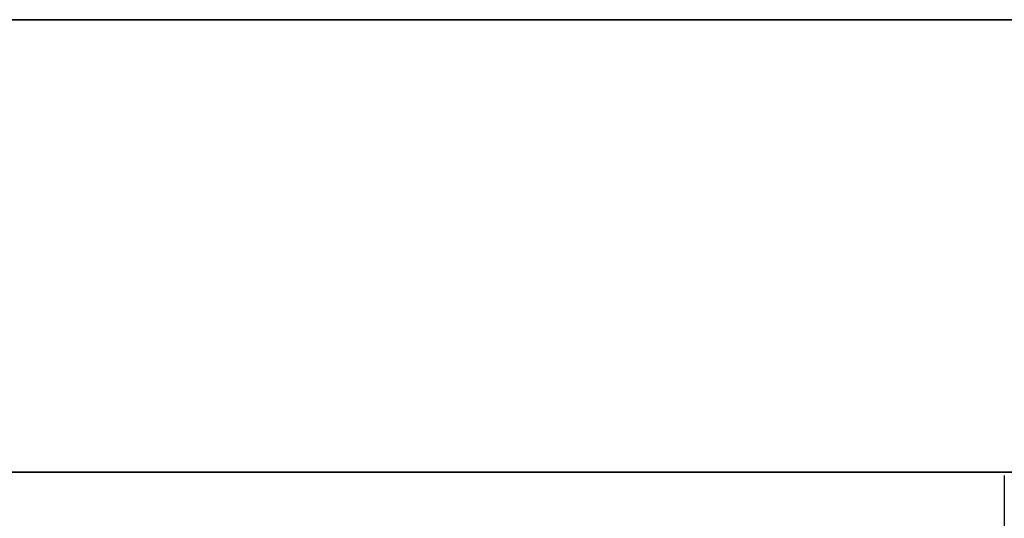
# Model space of a CAD drawing. Units: inches. Extents: x -86 to 2463, y -1058 to 68.
# Tile 8 of 17: x 49 to 69, y -304 to -294. Entities that reach past the tile are written whole.
import ezdxf

# ---------------------------------------------------------------- set-up
doc = ezdxf.new("R2010")
doc.units = ezdxf.units.IN
doc.header["$MEASUREMENT"] = 0
doc.layers.add('A-ANNO-DIMS', color=2, linetype='Continuous', lineweight=18)
doc.layers.add('A-WALL', color=7, linetype='Continuous', lineweight=35)
doc.styles.get("Standard").update_dxf_attribs({"font": 'arial.ttf'})
doc.dimstyles.get("Standard").update_dxf_attribs({"dimtxt": 0.18, "dimasz": 0.18, "dimexe": 0.18, "dimexo": 0.0625, "dimgap": 0.09, "dimtad": 0, "dimtih": 1, "dimtoh": 1, "dimdec": 4, "dimzin": 0, "dimdsep": 46, "dimtxsty": 'Standard', "dimcen": 0.09, "dimadec": 0, "dimazin": 0, "dimtfac": 1, "dimtdec": 4, "dimtofl": 0, "dimtmove": 0, "dimatfit": 3, "dimfxl": 1, "dimtolj": 1, "dimtzin": 0, "dimarcsym": 0})

# ---------------------------------------------------------------- blocks, each defined once
blk = doc.blocks.new('*D41')
at = {"layer": 'A-ANNO-DIMS', "color": 0, "lineweight": -2, "transparency": 16777216}
for p, q in [((15.761, -303.167), (15.761, -740.384)), ((68.889, -303.167), (68.889, -740.384)), ((15.941, -740.204), (41.931, -740.204)), ((68.709, -740.204), (42.719, -740.204))]:
    blk.add_line(p, q, dxfattribs=at)
at = {"layer": 'A-ANNO-DIMS', "color": 0, "transparency": 16777216}
for points in [[(15.941, -740.174), (15.941, -740.234), (15.761, -740.204)], [(68.709, -740.174), (68.709, -740.234), (68.889, -740.204)]]:
    blk.add_solid(points, dxfattribs=at)
at = {"layer": 'Defpoints', "color": 0, "transparency": 16777216}
for p in [(15.761, -303.104), (68.889, -303.104), (68.889, -740.204)]:
    blk.add_point(p, dxfattribs=at)
at = {"layer": 'A-ANNO-DIMS', "color": 0, "transparency": 16777216, "insert": (42.325, -740.204), "char_height": 0.18, "attachment_point": 5}
blk.add_mtext('\\A1;53.13', dxfattribs=at)
blk = doc.blocks.new('*D42')
at = {"layer": 'A-ANNO-DIMS', "color": 0, "lineweight": -2, "transparency": 16777216}
for p, q in [((68.889, -303.167), (68.889, -740.384)), ((104.261, -303.167), (104.261, -740.384)), ((69.069, -740.204), (86.181, -740.204)), ((104.081, -740.204), (86.969, -740.204))]:
    blk.add_line(p, q, dxfattribs=at)
at = {"layer": 'A-ANNO-DIMS', "color": 0, "transparency": 16777216}
for points in [[(69.069, -740.174), (69.069, -740.234), (68.889, -740.204)], [(104.081, -740.174), (104.081, -740.234), (104.261, -740.204)]]:
    blk.add_solid(points, dxfattribs=at)
at = {"layer": 'Defpoints', "color": 0, "transparency": 16777216}
for p in [(68.889, -303.104), (104.261, -303.104), (104.261, -740.204)]:
    blk.add_point(p, dxfattribs=at)
at = {"layer": 'A-ANNO-DIMS', "color": 0, "transparency": 16777216, "insert": (86.575, -740.204), "char_height": 0.18, "attachment_point": 5}
blk.add_mtext('\\A1;35.37', dxfattribs=at)

msp = doc.modelspace()

# ---------------------------------------------------------------- linework, layer by layer
at = {"layer": 'A-WALL'}
for p, q in [((183.761, -294.104), (24.761, -294.104)), ((377.846, -303.104), (15.761, -303.104))]:
    msp.add_line(p, q, dxfattribs=at)

# ---------------------------------------------------------------- dimensions: what is measured, and where the dimension line sits
at = {"layer": 'A-ANNO-DIMS'}
for base, p1, p2, picture, middle in [((68.889, -740.204), (15.761, -303.104), (68.889, -303.104), '*D41', (42.325, -740.204)), ((104.261, -740.204), (68.889, -303.104), (104.261, -303.104), '*D42', (86.575, -740.204))]:
    dim = msp.add_linear_dim(base=base, p1=p1, p2=p2, dimstyle='Standard', override={"dimdec": 2, "dimlfac": 1, "dimrnd": 0, "dimzin": 0, "dimdsep": 46, "dimlunit": 2}, dxfattribs=at)
    dim.commit()
    dim.dimension.update_dxf_attribs({"geometry": picture, "text_midpoint": middle})

doc.saveas('drawing.dxf')
